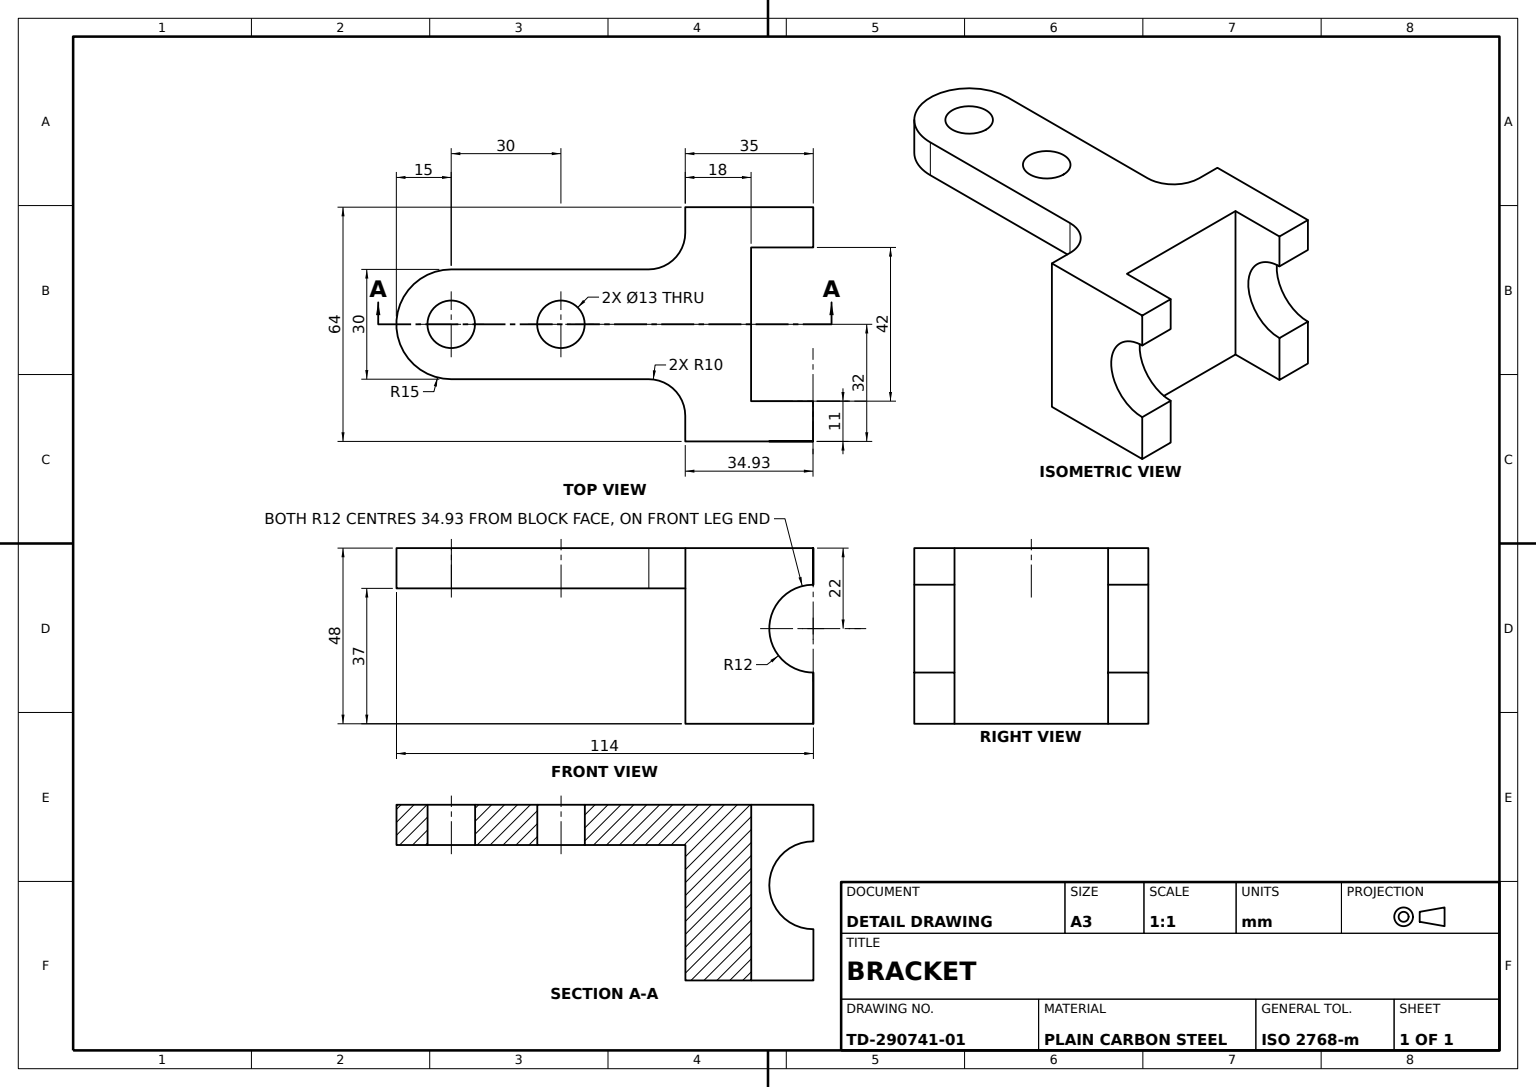
SolidWorks part; units mm, degrees
material "Plain Carbon Steel"
ref_plane "Front Plane" through (0, 0, 0) normal (0, 0, 1) x (1, 0, 0)
ref_plane "Top Plane" through (0, 0, 0) normal (0, 1, 0) x (1, 0, 0)
ref_plane "Right Plane" through (0, 0, 0) normal (1, 0, 0) x (0, 0, -1)
sketch "Plate Profile Sketch" plane through (0, 0, 0) normal (0, 1, 0) x (1, 0, 0)
  line L0 (0, 0) -> (0, 64) construction
  line L1 (-15, 0) -> (-15, 64)
  line L2 (15, 0) -> (15, 64)
  line L3 (-32, 64) -> (-15, 64)
  line L4 (32, 64) -> (32, 98.9341)
  line L5 (32, 98.9341) -> (21, 98.9341)
  line L6 (21, 98.9341) -> (21, 82)
  line L7 (21, 82) -> (-21, 82)
  line L8 (-21, 82) -> (-21, 99)
  line L9 (-21, 99) -> (-32, 99)
  line L10 (-32, 99) -> (-32, 64)
  line L11 (15, 64) -> (32, 64)
  arc A0 (-15, 0) -> (15, 0) centre (0, 0) ccw
  circle A2 centre (0, 0) radius 6.5
  circle A3 centre (0, 30) radius 6.5
  point P3 (0, 32)
  dimension "D2" = 15
  dimension "D3" = 13
  dimension "D4" = 13
  dimension "D1" = 64
  dimension "D5" = 30
  dimension "D6" = 64
  dimension "D7" = 42
  dimension "D8" = 11
  dimension "D9" = 11
  dimension "D10" = 35
  dimension "D11" = 18
  dimension "D12" = 32
  dimension "D13" = 34.9341
extrude "Mounting Plate 11mm" add sketch "Plate Profile Sketch" along normal blind 11
sketch "Support Block Sketch" plane through (0, 0, 0) normal (0, -1, 0) x (1, 0, 0)
  line L0 (-32, -64) -> (32, -64)
  line L1 (32, -64) -> (32, -98.9341)
  line L2 (32, -98.9341) -> (21, -98.9341)
  line L3 (21, -98.9341) -> (21, -82)
  line L4 (21, -82) -> (-21, -82)
  line L5 (-21, -82) -> (-21, -99)
  line L6 (-21, -99) -> (-32, -99)
  line L7 (-32, -99) -> (-32, -64)
extrude "Support Block 37mm" add sketch "Support Block Sketch" along normal blind 37
fillet "Fillet R10" radius 10 2 edges at (-15, 5.5, -64) (15, 5.5, -64)
sketch "Arm Hole Sketch" plane through (32, 0, 0) normal (1, 0, 0) x (0, 0, -1)
  line L0 (98.9341, 11) -> (98.9341, -37) construction
  line L1 (64, 11) -> (98.9341, 11) construction
  circle A0 centre (98.9341, -11) radius 12
  dimension "D1" = 24
  dimension "D2" = 22
extrude "Arm Hole" cut sketch "Arm Hole Sketch" against normal through all both and the other way through all
